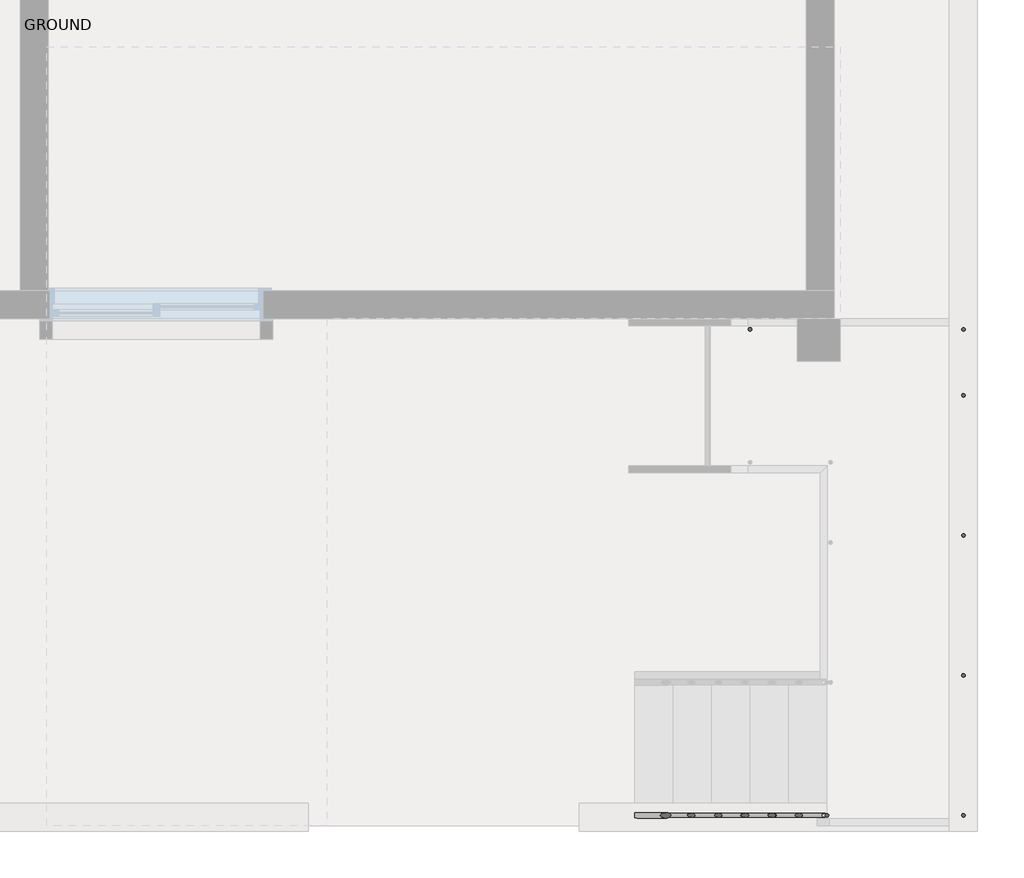
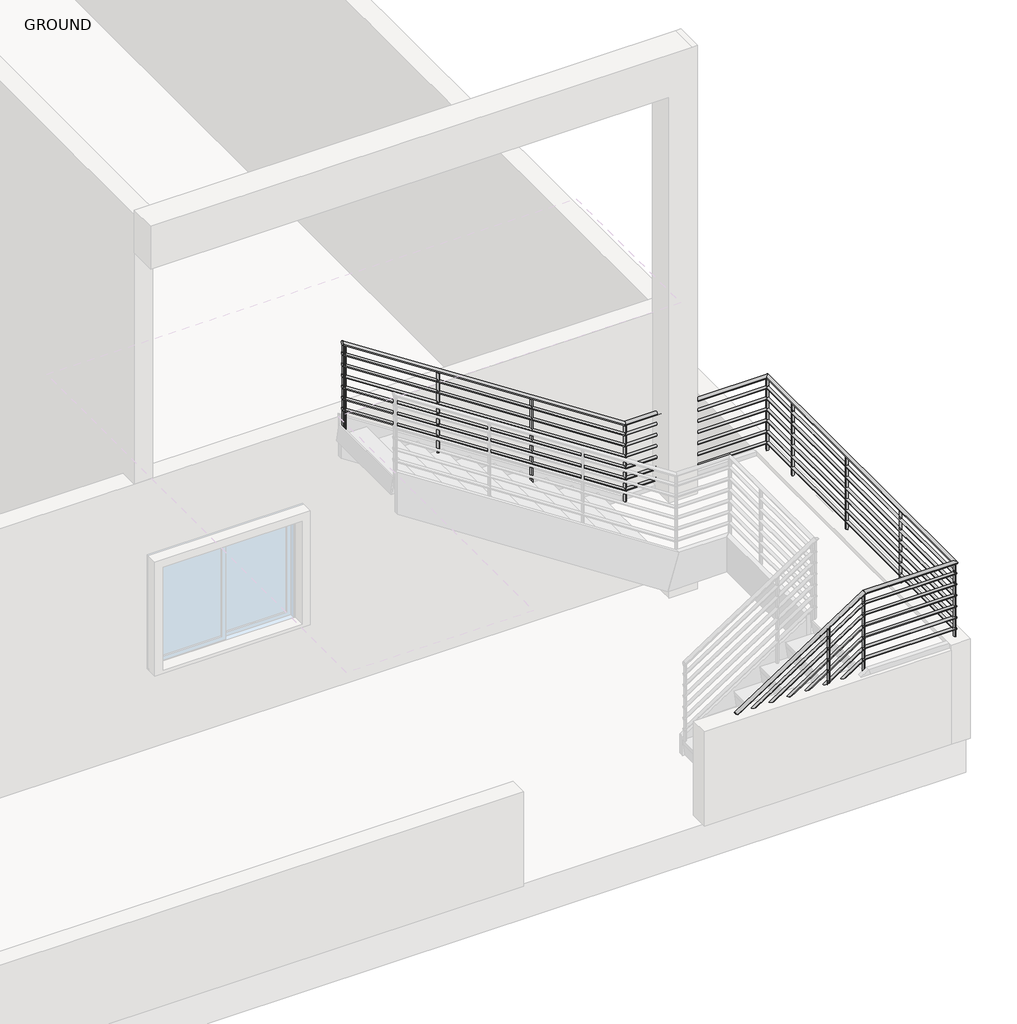
# One storey, part 2 of 4: 1 railing.
"""IFC4 building model written with IfcOpenShell, lengths in millimetres."""

from ifc_helpers import new_model, si_unit, point, frame, frame_2d, origin, place, context, project, spatial, circle_curve, ellipse_curve, trimmed, segment, composite_curve, outline, extrude, element, save
from ifc_brep_helpers import plane_surface, cylinder_surface, advanced_brep

model = new_model("IFC4")

# Units and contexts
model_context = context("Model", 3, world=origin())
ifc_project = project(units=[si_unit("LENGTHUNIT", "METRE", prefix="MILLI")], contexts=[model_context])

# Site, building, storey
site = spatial("IfcSite", under=ifc_project)
building = spatial("IfcBuilding", under=site)
storey = spatial("IfcBuildingStorey", under=building, Name="GROUND", Elevation=0.0)

# Railing
placement = place(None, origin())
element("IfcRailing", 1, ObjectType="900mm Pipe", at=placement, inside=storey, context=model_context, shape_type="SolidModel", body=[
    advanced_brep(
    [(11825.7864069, -3528.3536983, 1055.4188073), (11825.7864069, -3488.3536983, 1055.4188073), (13206.7303294, -3528.3536983, 1955.7647059), (13206.7303294, -3488.3536983, 1955.7647059), (14155.4121881, -3488.3536983, 1955.7647059), (14195.4121881, -3528.3536983, 1955.7647059), (14195.4121881, -17.2843256, 1955.7647059), (14155.4121881, -57.2843256, 1955.7647059), (12644.8424844, -17.2843256, 1955.7647059), (12644.8424844, -57.2843256, 1955.7647059), (9625.7864069, -17.2843256, 3924.1246897), (9625.7864069, -57.2843256, 3924.1246897)],
    [
        (0, 1, ellipse_curve(frame((11825.7864069, -3508.3536983, 1055.4188073), z_axis=(-1.0, 0.0, 0.0), x_axis=(0.0, 0.0, -1.0)), 23.8753103, 20.0)),
        (1, 0, ellipse_curve(frame((11825.7864069, -3508.3536983, 1055.4188073), z_axis=(-1.0, 0.0, 0.0), x_axis=(0.0, 0.0, -1.0)), 23.8753103, 20.0)),
        (0, 2),
        (2, 3, ellipse_curve(frame((13206.7303294, -3508.3536983, 1955.7647059), z_axis=(-0.9585628427581573, 0.0, -0.2848811620367351), x_axis=(0.28488116203673614, 0.0, -0.958562842758157)), 20.8645684, 20.0)),
        (3, 1),
        (3, 2, ellipse_curve(frame((13206.7303294, -3508.3536983, 1955.7647059), z_axis=(-0.9585628427581573, 0.0, -0.2848811620367351), x_axis=(0.28488116203673614, 0.0, -0.958562842758157)), 20.8645684, 20.0)),
        (4, 5, ellipse_curve(frame((14175.4121881, -3508.3536983, 1955.7647059), z_axis=(0.7071067811865513, 0.7071067811865438, 0.0), x_axis=(0.7071067811865439, -0.7071067811865512, 0.0)), 28.2842712, 20.0)),
        (5, 6),
        (6, 7, ellipse_curve(frame((14175.4121881, -37.2843256, 1955.7647059), z_axis=(0.7071067811865438, -0.7071067811865512, 0.0), x_axis=(-0.7071067811865512, -0.7071067811865438, 0.0)), 28.2842712, 20.0)),
        (7, 4),
        (5, 4, ellipse_curve(frame((14175.4121881, -3508.3536983, 1955.7647059), z_axis=(0.7071067811865513, 0.7071067811865438, 0.0), x_axis=(0.7071067811865439, -0.7071067811865512, 0.0)), 28.2842712, 20.0)),
        (7, 6, ellipse_curve(frame((14175.4121881, -37.2843256, 1955.7647059), z_axis=(0.7071067811865438, -0.7071067811865512, 0.0), x_axis=(-0.7071067811865512, -0.7071067811865438, 0.0)), 28.2842712, 20.0)),
        (6, 8),
        (8, 9, ellipse_curve(frame((12644.8424844, -37.2843256, 1955.7647059), z_axis=(0.9585628427581568, 0.0, -0.2848811620367359), x_axis=(0.2848811620367364, 0.0, 0.9585628427581568)), 20.8645684, 20.0)),
        (9, 7),
        (9, 8, ellipse_curve(frame((12644.8424844, -37.2843256, 1955.7647059), z_axis=(0.9585628427581568, 0.0, -0.2848811620367359), x_axis=(0.2848811620367364, 0.0, 0.9585628427581568)), 20.8645684, 20.0)),
        (10, 11, ellipse_curve(frame((9625.7864069, -37.2843256, 3924.1246897), z_axis=(-1.0, 0.0, 0.0), x_axis=(0.0, 0.0, -1.0)), 23.8753103, 20.0)),
        (11, 10, ellipse_curve(frame((9625.7864069, -37.2843256, 3924.1246897), z_axis=(-1.0, 0.0, 0.0), x_axis=(0.0, 0.0, -1.0)), 23.8753103, 20.0)),
        (8, 10),
        (11, 9),
        (2, 5),
        (4, 3),
    ],
    [
        plane_surface(frame((11825.7864069, -3508.3536983, 1079.2941176), z_axis=(-1.0, 0.0, 0.0), x_axis=(0.0, 1.0, 0.0))),
        cylinder_surface(frame((11836.7094668, -3508.3536983, 1062.5404087), z_axis=(-0.8376854470331991, 0.0, -0.5461529930603598), x_axis=(0.0, 1.0, 0.0)), 20.0),
        cylinder_surface(frame((14175.4121881, -3508.3536983, 1955.7647059), z_axis=(0.0, -1.0, 0.0), x_axis=(-1.0, 0.0, 0.0)), 20.0),
        cylinder_surface(frame((14175.4121881, -37.2843256, 1955.7647059), z_axis=(1.0, 0.0, 0.0), x_axis=(0.0, -1.0, 0.0)), 20.0),
        plane_surface(frame((9625.7864069, -37.2843256, 3948.0), z_axis=(-1.0, 0.0, 0.0), x_axis=(0.0, -1.0, 0.0))),
        cylinder_surface(frame((12639.863347, -37.2843256, 1959.0109969), z_axis=(0.8376854470331981, 0.0, -0.5461529930603612), x_axis=(0.0, -1.0, 0.0)), 20.0),
        cylinder_surface(frame((13200.7864069, -3508.3536983, 1955.7647059), z_axis=(-1.0, 0.0, 0.0), x_axis=(0.0, 1.0, 0.0)), 20.0),
    ],
    [
        (0, [[1, 2]]),
        (1, [[-1, 3, 4, 5]]),
        (1, [[-2, -5, 6, -3]]),
        (2, [[7, 8, 9, 10]]),
        (2, [[11, -10, 12, -8]]),
        (3, [[-9, 13, 14, 15]]),
        (3, [[-12, -15, 16, -13]]),
        (4, [[17, 18]]),
        (5, [[-14, 19, -18, 20]]),
        (5, [[-16, -20, -17, -19]]),
        (6, [[-4, 21, -7, 22]]),
        (6, [[-6, -22, -11, -21]]),
    ],
),
    advanced_brep(
    [(11825.7864069, -3493.3536983, 936.3876349), (11825.7864069, -3523.3536983, 936.3876349), (13205.2443488, -3493.3536983, 1835.7647059), (13205.2443488, -3523.3536983, 1835.7647059), (14160.4121881, -3493.3536983, 1835.7647059), (14190.4121881, -3523.3536983, 1835.7647059), (14160.4121881, -52.2843256, 1835.7647059), (14190.4121881, -22.2843256, 1835.7647059), (12646.328465, -52.2843256, 1835.7647059), (12646.328465, -22.2843256, 1835.7647059), (9625.7864069, -52.2843256, 3805.0935173), (9625.7864069, -22.2843256, 3805.0935173)],
    [
        (0, 1, ellipse_curve(frame((11825.7864069, -3508.3536983, 936.3876349), z_axis=(-1.0, 0.0, 0.0), x_axis=(0.0, 0.0, -1.0)), 17.9064827, 15.0)),
        (1, 0, ellipse_curve(frame((11825.7864069, -3508.3536983, 936.3876349), z_axis=(-1.0, 0.0, 0.0), x_axis=(0.0, 0.0, -1.0)), 17.9064827, 15.0)),
        (0, 2),
        (2, 3, ellipse_curve(frame((13205.2443488, -3508.3536983, 1835.7647059), z_axis=(-0.958562842758157, 0.0, -0.28488116203673564), x_axis=(0.28488116203673586, 0.0, -0.958562842758157)), 15.6484263, 15.0)),
        (3, 1),
        (3, 2, ellipse_curve(frame((13205.2443488, -3508.3536983, 1835.7647059), z_axis=(-0.958562842758157, 0.0, -0.28488116203673564), x_axis=(0.28488116203673586, 0.0, -0.958562842758157)), 15.6484263, 15.0)),
        (2, 4),
        (4, 5, ellipse_curve(frame((14175.4121881, -3508.3536983, 1835.7647059), z_axis=(-0.7071067811865513, -0.7071067811865438, 0.0), x_axis=(-0.7071067811865437, 0.7071067811865513, 0.0)), 21.2132034, 15.0)),
        (5, 3),
        (5, 4, ellipse_curve(frame((14175.4121881, -3508.3536983, 1835.7647059), z_axis=(-0.7071067811865513, -0.7071067811865438, 0.0), x_axis=(-0.7071067811865437, 0.7071067811865513, 0.0)), 21.2132034, 15.0)),
        (4, 6),
        (6, 7, ellipse_curve(frame((14175.4121881, -37.2843256, 1835.7647059), z_axis=(0.7071067811865438, -0.7071067811865512, 0.0), x_axis=(-0.7071067811865512, -0.7071067811865438, 0.0)), 21.2132034, 15.0)),
        (7, 5),
        (7, 6, ellipse_curve(frame((14175.4121881, -37.2843256, 1835.7647059), z_axis=(0.7071067811865438, -0.7071067811865512, 0.0), x_axis=(-0.7071067811865512, -0.7071067811865438, 0.0)), 21.2132034, 15.0)),
        (6, 8),
        (8, 9, ellipse_curve(frame((12646.328465, -37.2843256, 1835.7647059), z_axis=(0.958562842758157, 0.0, -0.2848811620367359), x_axis=(0.2848811620367357, 0.0, 0.958562842758157)), 15.6484263, 15.0)),
        (9, 7),
        (9, 8, ellipse_curve(frame((12646.328465, -37.2843256, 1835.7647059), z_axis=(0.958562842758157, 0.0, -0.2848811620367359), x_axis=(0.2848811620367357, 0.0, 0.958562842758157)), 15.6484263, 15.0)),
        (10, 11, ellipse_curve(frame((9625.7864069, -37.2843256, 3805.0935173), z_axis=(-1.0, 0.0, 0.0), x_axis=(0.0, 0.0, -1.0)), 17.9064827, 15.0)),
        (11, 10, ellipse_curve(frame((9625.7864069, -37.2843256, 3805.0935173), z_axis=(-1.0, 0.0, 0.0), x_axis=(0.0, 0.0, -1.0)), 17.9064827, 15.0)),
        (8, 10),
        (11, 9),
    ],
    [
        plane_surface(frame((11825.7864069, -3508.3536983, 954.2941176), z_axis=(-1.0, 0.0, 0.0), x_axis=(0.0, 1.0, 0.0))),
        cylinder_surface(frame((11833.9787018, -3508.3536983, 941.7288359), z_axis=(-0.8376854470331985, 0.0, -0.5461529930603609), x_axis=(0.0, -1.0, 0.0)), 15.0),
        cylinder_surface(frame((13200.7864069, -3508.3536983, 1835.7647059), z_axis=(-1.0, 0.0, 0.0), x_axis=(0.0, -1.0, 0.0)), 15.0),
        cylinder_surface(frame((14175.4121881, -3508.3536983, 1835.7647059), z_axis=(0.0, -1.0, 0.0), x_axis=(1.0, 0.0, 0.0)), 15.0),
        cylinder_surface(frame((14175.4121881, -37.2843256, 1835.7647059), z_axis=(1.0, 0.0, 0.0), x_axis=(0.0, 1.0, 0.0)), 15.0),
        plane_surface(frame((9625.7864069, -37.2843256, 3823.0), z_axis=(-1.0, 0.0, 0.0), x_axis=(0.0, -1.0, 0.0))),
        cylinder_surface(frame((12642.594112, -37.2843256, 1838.1994242), z_axis=(0.8376854470331982, 0.0, -0.5461529930603612), x_axis=(0.0, 1.0, 0.0)), 15.0),
    ],
    [
        (0, [[1, 2]]),
        (1, [[-1, 3, 4, 5]]),
        (1, [[-2, -5, 6, -3]]),
        (2, [[-4, 7, 8, 9]]),
        (2, [[-6, -9, 10, -7]]),
        (3, [[-8, 11, 12, 13]]),
        (3, [[-10, -13, 14, -11]]),
        (4, [[-12, 15, 16, 17]]),
        (4, [[-14, -17, 18, -15]]),
        (5, [[19, 20]]),
        (6, [[-16, 21, -20, 22]]),
        (6, [[-18, -22, -19, -21]]),
    ],
),
    advanced_brep(
    [(11825.7864069, -3493.3536983, 811.3876349), (11825.7864069, -3523.3536983, 811.3876349), (13205.2443488, -3493.3536983, 1710.7647059), (13205.2443488, -3523.3536983, 1710.7647059), (14160.4121881, -3493.3536983, 1710.7647059), (14190.4121881, -3523.3536983, 1710.7647059), (14160.4121881, -52.2843256, 1710.7647059), (14190.4121881, -22.2843256, 1710.7647059), (12646.328465, -52.2843256, 1710.7647059), (12646.328465, -22.2843256, 1710.7647059), (9625.7864069, -52.2843256, 3680.0935173), (9625.7864069, -22.2843256, 3680.0935173)],
    [
        (0, 1, ellipse_curve(frame((11825.7864069, -3508.3536983, 811.3876349), z_axis=(-1.0, 0.0, 0.0), x_axis=(0.0, 0.0, -1.0)), 17.9064827, 15.0)),
        (1, 0, ellipse_curve(frame((11825.7864069, -3508.3536983, 811.3876349), z_axis=(-1.0, 0.0, 0.0), x_axis=(0.0, 0.0, -1.0)), 17.9064827, 15.0)),
        (0, 2),
        (2, 3, ellipse_curve(frame((13205.2443488, -3508.3536983, 1710.7647059), z_axis=(-0.958562842758157, 0.0, -0.28488116203673564), x_axis=(0.28488116203673586, 0.0, -0.958562842758157)), 15.6484263, 15.0)),
        (3, 1),
        (3, 2, ellipse_curve(frame((13205.2443488, -3508.3536983, 1710.7647059), z_axis=(-0.958562842758157, 0.0, -0.28488116203673564), x_axis=(0.28488116203673586, 0.0, -0.958562842758157)), 15.6484263, 15.0)),
        (2, 4),
        (4, 5, ellipse_curve(frame((14175.4121881, -3508.3536983, 1710.7647059), z_axis=(-0.7071067811865513, -0.7071067811865438, 0.0), x_axis=(-0.7071067811865437, 0.7071067811865513, 0.0)), 21.2132034, 15.0)),
        (5, 3),
        (5, 4, ellipse_curve(frame((14175.4121881, -3508.3536983, 1710.7647059), z_axis=(-0.7071067811865513, -0.7071067811865438, 0.0), x_axis=(-0.7071067811865437, 0.7071067811865513, 0.0)), 21.2132034, 15.0)),
        (4, 6),
        (6, 7, ellipse_curve(frame((14175.4121881, -37.2843256, 1710.7647059), z_axis=(0.7071067811865438, -0.7071067811865512, 0.0), x_axis=(-0.7071067811865512, -0.7071067811865438, 0.0)), 21.2132034, 15.0)),
        (7, 5),
        (7, 6, ellipse_curve(frame((14175.4121881, -37.2843256, 1710.7647059), z_axis=(0.7071067811865438, -0.7071067811865512, 0.0), x_axis=(-0.7071067811865512, -0.7071067811865438, 0.0)), 21.2132034, 15.0)),
        (6, 8),
        (8, 9, ellipse_curve(frame((12646.328465, -37.2843256, 1710.7647059), z_axis=(0.9585628427581568, 0.0, -0.2848811620367359), x_axis=(0.28488116203673647, 0.0, 0.9585628427581567)), 15.6484263, 15.0)),
        (9, 7),
        (9, 8, ellipse_curve(frame((12646.328465, -37.2843256, 1710.7647059), z_axis=(0.9585628427581568, 0.0, -0.2848811620367359), x_axis=(0.28488116203673647, 0.0, 0.9585628427581567)), 15.6484263, 15.0)),
        (10, 11, ellipse_curve(frame((9625.7864069, -37.2843256, 3680.0935173), z_axis=(-1.0, 0.0, 0.0), x_axis=(0.0, 0.0, -1.0)), 17.9064827, 15.0)),
        (11, 10, ellipse_curve(frame((9625.7864069, -37.2843256, 3680.0935173), z_axis=(-1.0, 0.0, 0.0), x_axis=(0.0, 0.0, -1.0)), 17.9064827, 15.0)),
        (8, 10),
        (11, 9),
    ],
    [
        plane_surface(frame((11825.7864069, -3508.3536983, 829.2941176), z_axis=(-1.0, 0.0, 0.0), x_axis=(0.0, 1.0, 0.0))),
        cylinder_surface(frame((11833.9787018, -3508.3536983, 816.7288359), z_axis=(-0.8376854470331985, 0.0, -0.5461529930603609), x_axis=(0.0, -1.0, 0.0)), 15.0),
        cylinder_surface(frame((13200.7864069, -3508.3536983, 1710.7647059), z_axis=(-1.0, 0.0, 0.0), x_axis=(0.0, -1.0, 0.0)), 15.0),
        cylinder_surface(frame((14175.4121881, -3508.3536983, 1710.7647059), z_axis=(0.0, -1.0, 0.0), x_axis=(1.0, 0.0, 0.0)), 15.0),
        cylinder_surface(frame((14175.4121881, -37.2843256, 1710.7647059), z_axis=(1.0, 0.0, 0.0), x_axis=(0.0, 1.0, 0.0)), 15.0),
        plane_surface(frame((9625.7864069, -37.2843256, 3698.0), z_axis=(-1.0, 0.0, 0.0), x_axis=(0.0, -1.0, 0.0))),
        cylinder_surface(frame((12642.594112, -37.2843256, 1713.1994242), z_axis=(0.8376854470331981, 0.0, -0.5461529930603612), x_axis=(0.0, 1.0, 0.0)), 15.0),
    ],
    [
        (0, [[1, 2]]),
        (1, [[-1, 3, 4, 5]]),
        (1, [[-2, -5, 6, -3]]),
        (2, [[-4, 7, 8, 9]]),
        (2, [[-6, -9, 10, -7]]),
        (3, [[-8, 11, 12, 13]]),
        (3, [[-10, -13, 14, -11]]),
        (4, [[-12, 15, 16, 17]]),
        (4, [[-14, -17, 18, -15]]),
        (5, [[19, 20]]),
        (6, [[-16, 21, -20, 22]]),
        (6, [[-18, -22, -19, -21]]),
    ],
),
    advanced_brep(
    [(11825.7864069, -3493.3536983, 686.3876349), (11825.7864069, -3523.3536983, 686.3876349), (13205.2443488, -3493.3536983, 1585.7647059), (13205.2443488, -3523.3536983, 1585.7647059), (14160.4121881, -3493.3536983, 1585.7647059), (14190.4121881, -3523.3536983, 1585.7647059), (14160.4121881, -52.2843256, 1585.7647059), (14190.4121881, -22.2843256, 1585.7647059), (12646.328465, -52.2843256, 1585.7647059), (12646.328465, -22.2843256, 1585.7647059), (9625.7864069, -52.2843256, 3555.0935173), (9625.7864069, -22.2843256, 3555.0935173)],
    [
        (0, 1, ellipse_curve(frame((11825.7864069, -3508.3536983, 686.3876349), z_axis=(-1.0, 0.0, 0.0), x_axis=(0.0, 0.0, -1.0)), 17.9064827, 15.0)),
        (1, 0, ellipse_curve(frame((11825.7864069, -3508.3536983, 686.3876349), z_axis=(-1.0, 0.0, 0.0), x_axis=(0.0, 0.0, -1.0)), 17.9064827, 15.0)),
        (0, 2),
        (2, 3, ellipse_curve(frame((13205.2443488, -3508.3536983, 1585.7647059), z_axis=(-0.958562842758157, 0.0, -0.28488116203673564), x_axis=(0.28488116203673586, 0.0, -0.958562842758157)), 15.6484263, 15.0)),
        (3, 1),
        (3, 2, ellipse_curve(frame((13205.2443488, -3508.3536983, 1585.7647059), z_axis=(-0.958562842758157, 0.0, -0.28488116203673564), x_axis=(0.28488116203673586, 0.0, -0.958562842758157)), 15.6484263, 15.0)),
        (2, 4),
        (4, 5, ellipse_curve(frame((14175.4121881, -3508.3536983, 1585.7647059), z_axis=(-0.7071067811865513, -0.7071067811865438, 0.0), x_axis=(-0.7071067811865437, 0.7071067811865513, 0.0)), 21.2132034, 15.0)),
        (5, 3),
        (5, 4, ellipse_curve(frame((14175.4121881, -3508.3536983, 1585.7647059), z_axis=(-0.7071067811865513, -0.7071067811865438, 0.0), x_axis=(-0.7071067811865437, 0.7071067811865513, 0.0)), 21.2132034, 15.0)),
        (4, 6),
        (6, 7, ellipse_curve(frame((14175.4121881, -37.2843256, 1585.7647059), z_axis=(0.7071067811865438, -0.7071067811865512, 0.0), x_axis=(-0.7071067811865512, -0.7071067811865438, 0.0)), 21.2132034, 15.0)),
        (7, 5),
        (7, 6, ellipse_curve(frame((14175.4121881, -37.2843256, 1585.7647059), z_axis=(0.7071067811865438, -0.7071067811865512, 0.0), x_axis=(-0.7071067811865512, -0.7071067811865438, 0.0)), 21.2132034, 15.0)),
        (6, 8),
        (8, 9, ellipse_curve(frame((12646.328465, -37.2843256, 1585.7647059), z_axis=(0.958562842758157, 0.0, -0.28488116203673575), x_axis=(0.28488116203673586, 0.0, 0.958562842758157)), 15.6484263, 15.0)),
        (9, 7),
        (9, 8, ellipse_curve(frame((12646.328465, -37.2843256, 1585.7647059), z_axis=(0.958562842758157, 0.0, -0.28488116203673575), x_axis=(0.28488116203673586, 0.0, 0.958562842758157)), 15.6484263, 15.0)),
        (10, 11, ellipse_curve(frame((9625.7864069, -37.2843256, 3555.0935173), z_axis=(-1.0, 0.0, 0.0), x_axis=(0.0, 0.0, -1.0)), 17.9064827, 15.0)),
        (11, 10, ellipse_curve(frame((9625.7864069, -37.2843256, 3555.0935173), z_axis=(-1.0, 0.0, 0.0), x_axis=(0.0, 0.0, -1.0)), 17.9064827, 15.0)),
        (8, 10),
        (11, 9),
    ],
    [
        plane_surface(frame((11825.7864069, -3508.3536983, 704.2941176), z_axis=(-1.0, 0.0, 0.0), x_axis=(0.0, 1.0, 0.0))),
        cylinder_surface(frame((11833.9787018, -3508.3536983, 691.7288359), z_axis=(-0.8376854470331985, 0.0, -0.5461529930603609), x_axis=(0.0, -1.0, 0.0)), 15.0),
        cylinder_surface(frame((13200.7864069, -3508.3536983, 1585.7647059), z_axis=(-1.0, 0.0, 0.0), x_axis=(0.0, -1.0, 0.0)), 15.0),
        cylinder_surface(frame((14175.4121881, -3508.3536983, 1585.7647059), z_axis=(0.0, -1.0, 0.0), x_axis=(1.0, 0.0, 0.0)), 15.0),
        cylinder_surface(frame((14175.4121881, -37.2843256, 1585.7647059), z_axis=(1.0, 0.0, 0.0), x_axis=(0.0, 1.0, 0.0)), 15.0),
        plane_surface(frame((9625.7864069, -37.2843256, 3573.0), z_axis=(-1.0, 0.0, 0.0), x_axis=(0.0, -1.0, 0.0))),
        cylinder_surface(frame((12642.594112, -37.2843256, 1588.1994242), z_axis=(0.8376854470331982, 0.0, -0.546152993060361), x_axis=(0.0, 1.0, 0.0)), 15.0),
    ],
    [
        (0, [[1, 2]]),
        (1, [[-1, 3, 4, 5]]),
        (1, [[-2, -5, 6, -3]]),
        (2, [[-4, 7, 8, 9]]),
        (2, [[-6, -9, 10, -7]]),
        (3, [[-8, 11, 12, 13]]),
        (3, [[-10, -13, 14, -11]]),
        (4, [[-12, 15, 16, 17]]),
        (4, [[-14, -17, 18, -15]]),
        (5, [[19, 20]]),
        (6, [[-16, 21, -20, 22]]),
        (6, [[-18, -22, -19, -21]]),
    ],
),
    advanced_brep(
    [(11825.7864069, -3493.3536983, 561.3876349), (11825.7864069, -3523.3536983, 561.3876349), (13205.2443488, -3493.3536983, 1460.7647059), (13205.2443488, -3523.3536983, 1460.7647059), (14160.4121881, -3493.3536983, 1460.7647059), (14190.4121881, -3523.3536983, 1460.7647059), (14160.4121881, -52.2843256, 1460.7647059), (14190.4121881, -22.2843256, 1460.7647059), (12646.328465, -52.2843256, 1460.7647059), (12646.328465, -22.2843256, 1460.7647059), (9625.7864069, -52.2843256, 3430.0935173), (9625.7864069, -22.2843256, 3430.0935173)],
    [
        (0, 1, ellipse_curve(frame((11825.7864069, -3508.3536983, 561.3876349), z_axis=(-1.0, 0.0, 0.0), x_axis=(0.0, 0.0, -1.0)), 17.9064827, 15.0)),
        (1, 0, ellipse_curve(frame((11825.7864069, -3508.3536983, 561.3876349), z_axis=(-1.0, 0.0, 0.0), x_axis=(0.0, 0.0, -1.0)), 17.9064827, 15.0)),
        (0, 2),
        (2, 3, ellipse_curve(frame((13205.2443488, -3508.3536983, 1460.7647059), z_axis=(-0.958562842758157, 0.0, -0.28488116203673564), x_axis=(0.28488116203673586, 0.0, -0.958562842758157)), 15.6484263, 15.0)),
        (3, 1),
        (3, 2, ellipse_curve(frame((13205.2443488, -3508.3536983, 1460.7647059), z_axis=(-0.958562842758157, 0.0, -0.28488116203673564), x_axis=(0.28488116203673586, 0.0, -0.958562842758157)), 15.6484263, 15.0)),
        (2, 4),
        (4, 5, ellipse_curve(frame((14175.4121881, -3508.3536983, 1460.7647059), z_axis=(-0.7071067811865513, -0.7071067811865438, 0.0), x_axis=(-0.7071067811865437, 0.7071067811865513, 0.0)), 21.2132034, 15.0)),
        (5, 3),
        (5, 4, ellipse_curve(frame((14175.4121881, -3508.3536983, 1460.7647059), z_axis=(-0.7071067811865513, -0.7071067811865438, 0.0), x_axis=(-0.7071067811865437, 0.7071067811865513, 0.0)), 21.2132034, 15.0)),
        (4, 6),
        (6, 7, ellipse_curve(frame((14175.4121881, -37.2843256, 1460.7647059), z_axis=(0.7071067811865438, -0.7071067811865512, 0.0), x_axis=(-0.7071067811865512, -0.7071067811865438, 0.0)), 21.2132034, 15.0)),
        (7, 5),
        (7, 6, ellipse_curve(frame((14175.4121881, -37.2843256, 1460.7647059), z_axis=(0.7071067811865438, -0.7071067811865512, 0.0), x_axis=(-0.7071067811865512, -0.7071067811865438, 0.0)), 21.2132034, 15.0)),
        (6, 8),
        (8, 9, ellipse_curve(frame((12646.328465, -37.2843256, 1460.7647059), z_axis=(0.9585628427581568, 0.0, -0.2848811620367359), x_axis=(0.28488116203673647, 0.0, 0.9585628427581567)), 15.6484263, 15.0)),
        (9, 7),
        (9, 8, ellipse_curve(frame((12646.328465, -37.2843256, 1460.7647059), z_axis=(0.9585628427581568, 0.0, -0.2848811620367359), x_axis=(0.28488116203673647, 0.0, 0.9585628427581567)), 15.6484263, 15.0)),
        (10, 11, ellipse_curve(frame((9625.7864069, -37.2843256, 3430.0935173), z_axis=(-1.0, 0.0, 0.0), x_axis=(0.0, 0.0, -1.0)), 17.9064827, 15.0)),
        (11, 10, ellipse_curve(frame((9625.7864069, -37.2843256, 3430.0935173), z_axis=(-1.0, 0.0, 0.0), x_axis=(0.0, 0.0, -1.0)), 17.9064827, 15.0)),
        (8, 10),
        (11, 9),
    ],
    [
        plane_surface(frame((11825.7864069, -3508.3536983, 579.2941176), z_axis=(-1.0, 0.0, 0.0), x_axis=(0.0, 1.0, 0.0))),
        cylinder_surface(frame((11833.9787018, -3508.3536983, 566.7288359), z_axis=(-0.8376854470331985, 0.0, -0.5461529930603609), x_axis=(0.0, -1.0, 0.0)), 15.0),
        cylinder_surface(frame((13200.7864069, -3508.3536983, 1460.7647059), z_axis=(-1.0, 0.0, 0.0), x_axis=(0.0, -1.0, 0.0)), 15.0),
        cylinder_surface(frame((14175.4121881, -3508.3536983, 1460.7647059), z_axis=(0.0, -1.0, 0.0), x_axis=(1.0, 0.0, 0.0)), 15.0),
        cylinder_surface(frame((14175.4121881, -37.2843256, 1460.7647059), z_axis=(1.0, 0.0, 0.0), x_axis=(0.0, 1.0, 0.0)), 15.0),
        plane_surface(frame((9625.7864069, -37.2843256, 3448.0), z_axis=(-1.0, 0.0, 0.0), x_axis=(0.0, -1.0, 0.0))),
        cylinder_surface(frame((12642.594112, -37.2843256, 1463.1994242), z_axis=(0.8376854470331981, 0.0, -0.5461529930603612), x_axis=(0.0, 1.0, 0.0)), 15.0),
    ],
    [
        (0, [[1, 2]]),
        (1, [[-1, 3, 4, 5]]),
        (1, [[-2, -5, 6, -3]]),
        (2, [[-4, 7, 8, 9]]),
        (2, [[-6, -9, 10, -7]]),
        (3, [[-8, 11, 12, 13]]),
        (3, [[-10, -13, 14, -11]]),
        (4, [[-12, 15, 16, 17]]),
        (4, [[-14, -17, 18, -15]]),
        (5, [[19, 20]]),
        (6, [[-16, 21, -20, 22]]),
        (6, [[-18, -22, -19, -21]]),
    ],
),
    advanced_brep(
    [(11825.7864069, -3493.3536983, 436.3876349), (11825.7864069, -3523.3536983, 436.3876349), (13205.2443488, -3493.3536983, 1335.7647059), (13205.2443488, -3523.3536983, 1335.7647059), (14160.4121881, -3493.3536983, 1335.7647059), (14190.4121881, -3523.3536983, 1335.7647059), (14160.4121881, -52.2843256, 1335.7647059), (14190.4121881, -22.2843256, 1335.7647059), (12646.328465, -52.2843256, 1335.7647059), (12646.328465, -22.2843256, 1335.7647059), (9625.7864069, -52.2843256, 3305.0935173), (9625.7864069, -22.2843256, 3305.0935173)],
    [
        (0, 1, ellipse_curve(frame((11825.7864069, -3508.3536983, 436.3876349), z_axis=(-1.0, 0.0, 0.0), x_axis=(0.0, 0.0, -1.0)), 17.9064827, 15.0)),
        (1, 0, ellipse_curve(frame((11825.7864069, -3508.3536983, 436.3876349), z_axis=(-1.0, 0.0, 0.0), x_axis=(0.0, 0.0, -1.0)), 17.9064827, 15.0)),
        (0, 2),
        (2, 3, ellipse_curve(frame((13205.2443488, -3508.3536983, 1335.7647059), z_axis=(-0.958562842758157, 0.0, -0.28488116203673564), x_axis=(0.28488116203673586, 0.0, -0.958562842758157)), 15.6484263, 15.0)),
        (3, 1),
        (3, 2, ellipse_curve(frame((13205.2443488, -3508.3536983, 1335.7647059), z_axis=(-0.958562842758157, 0.0, -0.28488116203673564), x_axis=(0.28488116203673586, 0.0, -0.958562842758157)), 15.6484263, 15.0)),
        (2, 4),
        (4, 5, ellipse_curve(frame((14175.4121881, -3508.3536983, 1335.7647059), z_axis=(-0.7071067811865513, -0.7071067811865438, 0.0), x_axis=(-0.7071067811865437, 0.7071067811865513, 0.0)), 21.2132034, 15.0)),
        (5, 3),
        (5, 4, ellipse_curve(frame((14175.4121881, -3508.3536983, 1335.7647059), z_axis=(-0.7071067811865513, -0.7071067811865438, 0.0), x_axis=(-0.7071067811865437, 0.7071067811865513, 0.0)), 21.2132034, 15.0)),
        (4, 6),
        (6, 7, ellipse_curve(frame((14175.4121881, -37.2843256, 1335.7647059), z_axis=(0.7071067811865438, -0.7071067811865512, 0.0), x_axis=(-0.7071067811865512, -0.7071067811865438, 0.0)), 21.2132034, 15.0)),
        (7, 5),
        (7, 6, ellipse_curve(frame((14175.4121881, -37.2843256, 1335.7647059), z_axis=(0.7071067811865438, -0.7071067811865512, 0.0), x_axis=(-0.7071067811865512, -0.7071067811865438, 0.0)), 21.2132034, 15.0)),
        (6, 8),
        (8, 9, ellipse_curve(frame((12646.328465, -37.2843256, 1335.7647059), z_axis=(0.958562842758157, 0.0, -0.2848811620367359), x_axis=(0.2848811620367357, 0.0, 0.958562842758157)), 15.6484263, 15.0)),
        (9, 7),
        (9, 8, ellipse_curve(frame((12646.328465, -37.2843256, 1335.7647059), z_axis=(0.958562842758157, 0.0, -0.2848811620367359), x_axis=(0.2848811620367357, 0.0, 0.958562842758157)), 15.6484263, 15.0)),
        (10, 11, ellipse_curve(frame((9625.7864069, -37.2843256, 3305.0935173), z_axis=(-1.0, 0.0, 0.0), x_axis=(0.0, 0.0, -1.0)), 17.9064827, 15.0)),
        (11, 10, ellipse_curve(frame((9625.7864069, -37.2843256, 3305.0935173), z_axis=(-1.0, 0.0, 0.0), x_axis=(0.0, 0.0, -1.0)), 17.9064827, 15.0)),
        (8, 10),
        (11, 9),
    ],
    [
        plane_surface(frame((11825.7864069, -3508.3536983, 454.2941176), z_axis=(-1.0, 0.0, 0.0), x_axis=(0.0, 1.0, 0.0))),
        cylinder_surface(frame((11833.9787018, -3508.3536983, 441.7288359), z_axis=(-0.8376854470331985, 0.0, -0.5461529930603609), x_axis=(0.0, -1.0, 0.0)), 15.0),
        cylinder_surface(frame((13200.7864069, -3508.3536983, 1335.7647059), z_axis=(-1.0, 0.0, 0.0), x_axis=(0.0, -1.0, 0.0)), 15.0),
        cylinder_surface(frame((14175.4121881, -3508.3536983, 1335.7647059), z_axis=(0.0, -1.0, 0.0), x_axis=(1.0, 0.0, 0.0)), 15.0),
        cylinder_surface(frame((14175.4121881, -37.2843256, 1335.7647059), z_axis=(1.0, 0.0, 0.0), x_axis=(0.0, 1.0, 0.0)), 15.0),
        plane_surface(frame((9625.7864069, -37.2843256, 3323.0), z_axis=(-1.0, 0.0, 0.0), x_axis=(0.0, -1.0, 0.0))),
        cylinder_surface(frame((12642.594112, -37.2843256, 1338.1994242), z_axis=(0.8376854470331982, 0.0, -0.5461529930603612), x_axis=(0.0, 1.0, 0.0)), 15.0),
    ],
    [
        (0, [[1, 2]]),
        (1, [[-1, 3, 4, 5]]),
        (1, [[-2, -5, 6, -3]]),
        (2, [[-4, 7, 8, 9]]),
        (2, [[-6, -9, 10, -7]]),
        (3, [[-8, 11, 12, 13]]),
        (3, [[-10, -13, 14, -11]]),
        (4, [[-12, 15, 16, 17]]),
        (4, [[-14, -17, 18, -15]]),
        (5, [[19, 20]]),
        (6, [[-16, 21, -20, 22]]),
        (6, [[-18, -22, -19, -21]]),
    ],
),
    advanced_brep(
    [(11825.7864069, -3493.3536983, 311.3876349), (11825.7864069, -3523.3536983, 311.3876349), (13205.2443488, -3493.3536983, 1210.7647059), (13205.2443488, -3523.3536983, 1210.7647059), (14160.4121881, -3493.3536983, 1210.7647059), (14190.4121881, -3523.3536983, 1210.7647059), (14160.4121881, -52.2843256, 1210.7647059), (14190.4121881, -22.2843256, 1210.7647059), (12646.328465, -52.2843256, 1210.7647059), (12646.328465, -22.2843256, 1210.7647059), (9625.7864069, -52.2843256, 3180.0935173), (9625.7864069, -22.2843256, 3180.0935173)],
    [
        (0, 1, ellipse_curve(frame((11825.7864069, -3508.3536983, 311.3876349), z_axis=(-1.0, 0.0, 0.0), x_axis=(0.0, 0.0, -1.0)), 17.9064827, 15.0)),
        (1, 0, ellipse_curve(frame((11825.7864069, -3508.3536983, 311.3876349), z_axis=(-1.0, 0.0, 0.0), x_axis=(0.0, 0.0, -1.0)), 17.9064827, 15.0)),
        (0, 2),
        (2, 3, ellipse_curve(frame((13205.2443488, -3508.3536983, 1210.7647059), z_axis=(-0.958562842758157, 0.0, -0.28488116203673564), x_axis=(0.28488116203673586, 0.0, -0.958562842758157)), 15.6484263, 15.0)),
        (3, 1),
        (3, 2, ellipse_curve(frame((13205.2443488, -3508.3536983, 1210.7647059), z_axis=(-0.958562842758157, 0.0, -0.28488116203673564), x_axis=(0.28488116203673586, 0.0, -0.958562842758157)), 15.6484263, 15.0)),
        (2, 4),
        (4, 5, ellipse_curve(frame((14175.4121881, -3508.3536983, 1210.7647059), z_axis=(-0.7071067811865513, -0.7071067811865438, 0.0), x_axis=(-0.7071067811865437, 0.7071067811865513, 0.0)), 21.2132034, 15.0)),
        (5, 3),
        (5, 4, ellipse_curve(frame((14175.4121881, -3508.3536983, 1210.7647059), z_axis=(-0.7071067811865513, -0.7071067811865438, 0.0), x_axis=(-0.7071067811865437, 0.7071067811865513, 0.0)), 21.2132034, 15.0)),
        (4, 6),
        (6, 7, ellipse_curve(frame((14175.4121881, -37.2843256, 1210.7647059), z_axis=(0.7071067811865438, -0.7071067811865512, 0.0), x_axis=(-0.7071067811865512, -0.7071067811865438, 0.0)), 21.2132034, 15.0)),
        (7, 5),
        (7, 6, ellipse_curve(frame((14175.4121881, -37.2843256, 1210.7647059), z_axis=(0.7071067811865438, -0.7071067811865512, 0.0), x_axis=(-0.7071067811865512, -0.7071067811865438, 0.0)), 21.2132034, 15.0)),
        (6, 8),
        (8, 9, ellipse_curve(frame((12646.328465, -37.2843256, 1210.7647059), z_axis=(0.9585628427581568, 0.0, -0.2848811620367359), x_axis=(0.28488116203673647, 0.0, 0.9585628427581567)), 15.6484263, 15.0)),
        (9, 7),
        (9, 8, ellipse_curve(frame((12646.328465, -37.2843256, 1210.7647059), z_axis=(0.9585628427581568, 0.0, -0.2848811620367359), x_axis=(0.28488116203673647, 0.0, 0.9585628427581567)), 15.6484263, 15.0)),
        (10, 11, ellipse_curve(frame((9625.7864069, -37.2843256, 3180.0935173), z_axis=(-1.0, 0.0, 0.0), x_axis=(0.0, 0.0, -1.0)), 17.9064827, 15.0)),
        (11, 10, ellipse_curve(frame((9625.7864069, -37.2843256, 3180.0935173), z_axis=(-1.0, 0.0, 0.0), x_axis=(0.0, 0.0, -1.0)), 17.9064827, 15.0)),
        (8, 10),
        (11, 9),
    ],
    [
        plane_surface(frame((11825.7864069, -3508.3536983, 329.2941176), z_axis=(-1.0, 0.0, 0.0), x_axis=(0.0, 1.0, 0.0))),
        cylinder_surface(frame((11833.9787018, -3508.3536983, 316.7288359), z_axis=(-0.8376854470331985, 0.0, -0.5461529930603609), x_axis=(0.0, -1.0, 0.0)), 15.0),
        cylinder_surface(frame((13200.7864069, -3508.3536983, 1210.7647059), z_axis=(-1.0, 0.0, 0.0), x_axis=(0.0, -1.0, 0.0)), 15.0),
        cylinder_surface(frame((14175.4121881, -3508.3536983, 1210.7647059), z_axis=(0.0, -1.0, 0.0), x_axis=(1.0, 0.0, 0.0)), 15.0),
        cylinder_surface(frame((14175.4121881, -37.2843256, 1210.7647059), z_axis=(1.0, 0.0, 0.0), x_axis=(0.0, 1.0, 0.0)), 15.0),
        plane_surface(frame((9625.7864069, -37.2843256, 3198.0), z_axis=(-1.0, 0.0, 0.0), x_axis=(0.0, -1.0, 0.0))),
        cylinder_surface(frame((12642.594112, -37.2843256, 1213.1994242), z_axis=(0.8376854470331981, 0.0, -0.5461529930603612), x_axis=(0.0, 1.0, 0.0)), 15.0),
    ],
    [
        (0, [[1, 2]]),
        (1, [[-1, 3, 4, 5]]),
        (1, [[-2, -5, 6, -3]]),
        (2, [[-4, 7, 8, 9]]),
        (2, [[-6, -9, 10, -7]]),
        (3, [[-8, 11, 12, 13]]),
        (3, [[-10, -13, 14, -11]]),
        (4, [[-12, 15, 16, 17]]),
        (4, [[-14, -17, 18, -15]]),
        (5, [[19, 20]]),
        (6, [[-16, 21, -20, 22]]),
        (6, [[-18, -22, -19, -21]]),
    ],
),
    advanced_brep(
    [(9650.7864069, -24.7843256, 3883.9499141), (9650.7864069, -24.7843256, 2868.7058824), (9650.7864069, -49.7843256, 2868.7058824), (9650.7864069, -49.7843256, 3883.9499141)],
    [
        (0, 1),
        (1, 2, circle_curve(frame((9650.7864069, -37.2843256, 2868.7058824), z_axis=(0.0, 0.0, 1.0), x_axis=(0.0, -1.0, 0.0)), 12.5)),
        (2, 3),
        (3, 0, ellipse_curve(frame((9650.7864069, -37.2843256, 3883.9499141), z_axis=(-0.546152993060361, 0.0, -0.8376854470331982), x_axis=(-0.8376854470331982, 0.0, 0.546152993060361)), 14.922069, 12.5)),
        (0, 3, ellipse_curve(frame((9650.7864069, -37.2843256, 3883.9499141), z_axis=(-0.546152993060361, 0.0, -0.8376854470331982), x_axis=(-0.8376854470331982, 0.0, 0.546152993060361)), 14.922069, 12.5)),
        (2, 1, circle_curve(frame((9650.7864069, -37.2843256, 2868.7058824), z_axis=(0.0, 0.0, 1.0), x_axis=(0.0, -1.0, 0.0)), 12.5)),
    ],
    [
        cylinder_surface(frame((9650.7864069, -37.2843256, 2768.7058824), z_axis=(0.0, 0.0, 1.0), x_axis=(0.0, -1.0, 0.0)), 12.5),
        plane_surface(frame((9625.7864069, -62.2843256, 3900.2493794), z_axis=(0.546152993060361, 0.0, 0.8376854470331982), x_axis=(0.0, 1.0, 0.0))),
        plane_surface(frame((9675.7864069, -62.2843256, 2868.7058824), z_axis=(0.0, 0.0, -1.0), x_axis=(0.0, 1.0, 0.0))),
    ],
    [
        (0, [[1, 2, 3, 4]]),
        (0, [[-1, 5, -3, 6]]),
        (1, [[-4, -5]]),
        (2, [[-2, -6]]),
    ],
),
    advanced_brep(
    [(10650.7864069, -24.7843256, 3231.9713045), (10650.7864069, -24.7843256, 2330.8235294), (10650.7864069, -49.7843256, 2330.8235294), (10650.7864069, -49.7843256, 3231.9713045)],
    [
        (0, 1),
        (1, 2, circle_curve(frame((10650.7864069, -37.2843256, 2330.8235294), z_axis=(0.0, 0.0, 1.0), x_axis=(0.0, -1.0, 0.0)), 12.5)),
        (2, 3),
        (3, 0, ellipse_curve(frame((10650.7864069, -37.2843256, 3231.9713045), z_axis=(-0.5461529930603595, 0.0, -0.8376854470331992), x_axis=(-0.8376854470331992, 0.0, 0.5461529930603595)), 14.922069, 12.5)),
        (0, 3, ellipse_curve(frame((10650.7864069, -37.2843256, 3231.9713045), z_axis=(-0.5461529930603595, 0.0, -0.8376854470331992), x_axis=(-0.8376854470331992, 0.0, 0.5461529930603595)), 14.922069, 12.5)),
        (2, 1, circle_curve(frame((10650.7864069, -37.2843256, 2330.8235294), z_axis=(0.0, 0.0, 1.0), x_axis=(0.0, -1.0, 0.0)), 12.5)),
    ],
    [
        cylinder_surface(frame((10650.7864069, -37.2843256, 2230.8235294), z_axis=(0.0, 0.0, 1.0), x_axis=(0.0, -1.0, 0.0)), 12.5),
        plane_surface(frame((10625.7864069, -62.2843256, 3248.2707697), z_axis=(0.5461529930603595, 0.0, 0.8376854470331992), x_axis=(0.0, 1.0, 0.0))),
        plane_surface(frame((10675.7864069, -62.2843256, 2330.8235294), z_axis=(0.0, 0.0, -1.0), x_axis=(0.0, 1.0, 0.0))),
    ],
    [
        (0, [[1, 2, 3, 4]]),
        (0, [[-1, 5, -3, 6]]),
        (1, [[-4, -5]]),
        (2, [[-2, -6]]),
    ],
),
    advanced_brep(
    [(11650.7864069, -24.7843256, 2579.9926949), (11650.7864069, -24.7843256, 1613.6470588), (11650.7864069, -49.7843256, 1613.6470588), (11650.7864069, -49.7843256, 2579.9926949)],
    [
        (0, 1),
        (1, 2, circle_curve(frame((11650.7864069, -37.2843256, 1613.6470588), z_axis=(0.0, 0.0, 1.0), x_axis=(0.0, -1.0, 0.0)), 12.5)),
        (2, 3),
        (3, 0, ellipse_curve(frame((11650.7864069, -37.2843256, 2579.9926949), z_axis=(-0.5461529930603595, 0.0, -0.8376854470331992), x_axis=(-0.8376854470331992, 0.0, 0.5461529930603595)), 14.922069, 12.5)),
        (0, 3, ellipse_curve(frame((11650.7864069, -37.2843256, 2579.9926949), z_axis=(-0.5461529930603595, 0.0, -0.8376854470331992), x_axis=(-0.8376854470331992, 0.0, 0.5461529930603595)), 14.922069, 12.5)),
        (2, 1, circle_curve(frame((11650.7864069, -37.2843256, 1613.6470588), z_axis=(0.0, 0.0, 1.0), x_axis=(0.0, -1.0, 0.0)), 12.5)),
    ],
    [
        cylinder_surface(frame((11650.7864069, -37.2843256, 1513.6470588), z_axis=(0.0, 0.0, 1.0), x_axis=(0.0, -1.0, 0.0)), 12.5),
        plane_surface(frame((11625.7864069, -62.2843256, 2596.2921601), z_axis=(0.5461529930603595, 0.0, 0.8376854470331992), x_axis=(0.0, 1.0, 0.0))),
        plane_surface(frame((11675.7864069, -62.2843256, 1613.6470588), z_axis=(0.0, 0.0, -1.0), x_axis=(0.0, 1.0, 0.0))),
    ],
    [
        (0, [[1, 2, 3, 4]]),
        (0, [[-1, 5, -3, 6]]),
        (1, [[-4, -5]]),
        (2, [[-2, -6]]),
    ],
),
    extrude(outline(composite_curve([segment(trimmed(circle_curve(frame_2d((13175.4121881, -37.2843256)), 12.5), [point((13175.4121881, -49.7843256))], [point((13175.4121881, -24.7843256))], False, "CARTESIAN"), True, "CONTINUOUS"), segment(trimmed(circle_curve(frame_2d((13175.4121881, -37.2843256)), 12.5), [point((13175.4121881, -24.7843256))], [point((13175.4121881, -49.7843256))], False, "CARTESIAN"), True, "CONTINUOUS")], self_intersect=False)), frame((0.0, 0.0, 1075.7647059), z_axis=(0.0, 0.0, 1.0), x_axis=(1.0, 0.0, 0.0)), (0.0, 0.0, 1.0), 860.0),
    extrude(outline(composite_curve([segment(trimmed(circle_curve(frame_2d((14175.4121881, -508.3536983)), 12.5), [point((14162.9121881, -508.3536983))], [point((14187.9121881, -508.3536983))], False, "CARTESIAN"), True, "CONTINUOUS"), segment(trimmed(circle_curve(frame_2d((14175.4121881, -508.3536983)), 12.5), [point((14187.9121881, -508.3536983))], [point((14162.9121881, -508.3536983))], False, "CARTESIAN"), True, "CONTINUOUS")], self_intersect=False)), frame((0.0, 0.0, 1075.7647059), z_axis=(0.0, 0.0, 1.0), x_axis=(1.0, 0.0, 0.0)), (0.0, 0.0, 1.0), 860.0),
    extrude(outline(composite_curve([segment(trimmed(circle_curve(frame_2d((14175.4121881, -1508.3536983)), 12.5), [point((14162.9121881, -1508.3536983))], [point((14187.9121881, -1508.3536983))], False, "CARTESIAN"), True, "CONTINUOUS"), segment(trimmed(circle_curve(frame_2d((14175.4121881, -1508.3536983)), 12.5), [point((14187.9121881, -1508.3536983))], [point((14162.9121881, -1508.3536983))], False, "CARTESIAN"), True, "CONTINUOUS")], self_intersect=False)), frame((0.0, 0.0, 1075.7647059), z_axis=(0.0, 0.0, 1.0), x_axis=(1.0, 0.0, 0.0)), (0.0, 0.0, 1.0), 860.0),
    extrude(outline(composite_curve([segment(trimmed(circle_curve(frame_2d((14175.4121881, -2508.3536983)), 12.5), [point((14162.9121881, -2508.3536983))], [point((14187.9121881, -2508.3536983))], False, "CARTESIAN"), True, "CONTINUOUS"), segment(trimmed(circle_curve(frame_2d((14175.4121881, -2508.3536983)), 12.5), [point((14187.9121881, -2508.3536983))], [point((14162.9121881, -2508.3536983))], False, "CARTESIAN"), True, "CONTINUOUS")], self_intersect=False)), frame((0.0, 0.0, 1075.7647059), z_axis=(0.0, 0.0, 1.0), x_axis=(1.0, 0.0, 0.0)), (0.0, 0.0, 1.0), 860.0),
    advanced_brep(
    [(12825.7864069, -3520.8536983, 1683.5221066), (12825.7864069, -3520.8536983, 717.1764706), (12825.7864069, -3495.8536983, 717.1764706), (12825.7864069, -3495.8536983, 1683.5221066)],
    [
        (0, 1),
        (1, 2, circle_curve(frame((12825.7864069, -3508.3536983, 717.1764706), z_axis=(0.0, 0.0, 1.0), x_axis=(0.0, 1.0, 0.0)), 12.5)),
        (2, 3),
        (3, 0, ellipse_curve(frame((12825.7864069, -3508.3536983, 1683.5221066), z_axis=(0.5461529930603595, 0.0, -0.8376854470331992), x_axis=(0.8376854470331992, 0.0, 0.5461529930603595)), 14.922069, 12.5)),
        (0, 3, ellipse_curve(frame((12825.7864069, -3508.3536983, 1683.5221066), z_axis=(0.5461529930603595, 0.0, -0.8376854470331992), x_axis=(0.8376854470331992, 0.0, 0.5461529930603595)), 14.922069, 12.5)),
        (2, 1, circle_curve(frame((12825.7864069, -3508.3536983, 717.1764706), z_axis=(0.0, 0.0, 1.0), x_axis=(0.0, 1.0, 0.0)), 12.5)),
    ],
    [
        cylinder_surface(frame((12825.7864069, -3508.3536983, 617.1764706), z_axis=(0.0, 0.0, 1.0), x_axis=(0.0, 1.0, 0.0)), 12.5),
        plane_surface(frame((12850.7864069, -3483.3536983, 1699.8215719), z_axis=(-0.5461529930603595, 0.0, 0.8376854470331992), x_axis=(0.0, -1.0, 0.0))),
        plane_surface(frame((12800.7864069, -3483.3536983, 717.1764706), z_axis=(0.0, 0.0, -1.0), x_axis=(0.0, -1.0, 0.0))),
    ],
    [
        (0, [[1, 2, 3, 4]]),
        (0, [[-1, 5, -3, 6]]),
        (1, [[-4, -5]]),
        (2, [[-2, -6]]),
    ],
),
    extrude(outline(composite_curve([segment(trimmed(circle_curve(frame_2d((12650.7864069, -37.2843256)), 12.5), [point((12650.7864069, -49.7843256))], [point((12650.7864069, -24.7843256))], False, "CARTESIAN"), True, "CONTINUOUS"), segment(trimmed(circle_curve(frame_2d((12650.7864069, -37.2843256)), 12.5), [point((12650.7864069, -24.7843256))], [point((12650.7864069, -49.7843256))], False, "CARTESIAN"), True, "CONTINUOUS")], self_intersect=False)), frame((0.0, 0.0, 1075.7647059), z_axis=(0.0, 0.0, 1.0), x_axis=(1.0, 0.0, 0.0)), (0.0, 0.0, 1.0), 860.0),
    extrude(outline(composite_curve([segment(trimmed(circle_curve(frame_2d((14175.4121881, -37.2843256)), 12.5), [point((14162.9121881, -37.2843256))], [point((14187.9121881, -37.2843256))], False, "CARTESIAN"), True, "CONTINUOUS"), segment(trimmed(circle_curve(frame_2d((14175.4121881, -37.2843256)), 12.5), [point((14187.9121881, -37.2843256))], [point((14162.9121881, -37.2843256))], False, "CARTESIAN"), True, "CONTINUOUS")], self_intersect=False)), frame((0.0, 0.0, 1075.7647059), z_axis=(0.0, 0.0, 1.0), x_axis=(1.0, 0.0, 0.0)), (0.0, 0.0, 1.0), 860.0),
    extrude(outline(composite_curve([segment(trimmed(circle_curve(frame_2d((14175.4121881, -3508.3536983)), 12.5), [point((14175.4121881, -3495.8536983))], [point((14175.4121881, -3520.8536983))], False, "CARTESIAN"), True, "CONTINUOUS"), segment(trimmed(circle_curve(frame_2d((14175.4121881, -3508.3536983)), 12.5), [point((14175.4121881, -3520.8536983))], [point((14175.4121881, -3495.8536983))], False, "CARTESIAN"), True, "CONTINUOUS")], self_intersect=False)), frame((0.0, 0.0, 1075.7647059), z_axis=(0.0, 0.0, 1.0), x_axis=(1.0, 0.0, 0.0)), (0.0, 0.0, 1.0), 860.0),
    extrude(outline(composite_curve([segment(trimmed(circle_curve(frame_2d((13200.7864069, -3508.3536983)), 12.5), [point((13200.7864069, -3495.8536983))], [point((13200.7864069, -3520.8536983))], False, "CARTESIAN"), True, "CONTINUOUS"), segment(trimmed(circle_curve(frame_2d((13200.7864069, -3508.3536983)), 12.5), [point((13200.7864069, -3520.8536983))], [point((13200.7864069, -3495.8536983))], False, "CARTESIAN"), True, "CONTINUOUS")], self_intersect=False)), frame((0.0, 0.0, 1075.7647059), z_axis=(0.0, 0.0, 1.0), x_axis=(1.0, 0.0, 0.0)), (0.0, 0.0, 1.0), 860.0),
    advanced_brep(
    [(9638.2864069, -24.7843256, 3892.0996467), (9638.2864069, -24.7843256, 2868.7058824), (9638.2864069, -49.7843256, 2868.7058824), (9638.2864069, -49.7843256, 3892.0996467)],
    [
        (0, 1),
        (1, 2, circle_curve(frame((9638.2864069, -37.2843256, 2868.7058824), z_axis=(0.0, 0.0, 1.0), x_axis=(0.0, -1.0, 0.0)), 12.5)),
        (2, 3),
        (3, 0, ellipse_curve(frame((9638.2864069, -37.2843256, 3892.0996467), z_axis=(-0.546152993060361, 0.0, -0.8376854470331982), x_axis=(-0.8376854470331982, 0.0, 0.546152993060361)), 14.922069, 12.5)),
        (0, 3, ellipse_curve(frame((9638.2864069, -37.2843256, 3892.0996467), z_axis=(-0.546152993060361, 0.0, -0.8376854470331982), x_axis=(-0.8376854470331982, 0.0, 0.546152993060361)), 14.922069, 12.5)),
        (2, 1, circle_curve(frame((9638.2864069, -37.2843256, 2868.7058824), z_axis=(0.0, 0.0, 1.0), x_axis=(0.0, -1.0, 0.0)), 12.5)),
    ],
    [
        cylinder_surface(frame((9638.2864069, -37.2843256, 2768.7058824), z_axis=(0.0, 0.0, 1.0), x_axis=(0.0, -1.0, 0.0)), 12.5),
        plane_surface(frame((9613.2864069, -62.2843256, 3908.399112), z_axis=(0.546152993060361, 0.0, 0.8376854470331982), x_axis=(0.0, 1.0, 0.0))),
        plane_surface(frame((9663.2864069, -62.2843256, 2868.7058824), z_axis=(0.0, 0.0, -1.0), x_axis=(0.0, 1.0, 0.0))),
    ],
    [
        (0, [[1, 2, 3, 4]]),
        (0, [[-1, 5, -3, 6]]),
        (1, [[-4, -5]]),
        (2, [[-2, -6]]),
    ],
),
    advanced_brep(
    [(11838.2864069, -3520.8536983, 1039.6932296), (11838.2864069, -3520.8536983, 179.2941176), (11838.2864069, -3495.8536983, 179.2941176), (11838.2864069, -3495.8536983, 1039.6932296)],
    [
        (0, 1),
        (1, 2, circle_curve(frame((11838.2864069, -3508.3536983, 179.2941176), z_axis=(0.0, 0.0, 1.0), x_axis=(0.0, 1.0, 0.0)), 12.5)),
        (2, 3),
        (3, 0, ellipse_curve(frame((11838.2864069, -3508.3536983, 1039.6932296), z_axis=(0.5461529930603595, 0.0, -0.8376854470331992), x_axis=(0.8376854470331992, 0.0, 0.5461529930603595)), 14.922069, 12.5)),
        (0, 3, ellipse_curve(frame((11838.2864069, -3508.3536983, 1039.6932296), z_axis=(0.5461529930603595, 0.0, -0.8376854470331992), x_axis=(0.8376854470331992, 0.0, 0.5461529930603595)), 14.922069, 12.5)),
        (2, 1, circle_curve(frame((11838.2864069, -3508.3536983, 179.2941176), z_axis=(0.0, 0.0, 1.0), x_axis=(0.0, 1.0, 0.0)), 12.5)),
    ],
    [
        cylinder_surface(frame((11838.2864069, -3508.3536983, 79.2941176), z_axis=(0.0, 0.0, 1.0), x_axis=(0.0, 1.0, 0.0)), 12.5),
        plane_surface(frame((11863.2864069, -3483.3536983, 1055.9926949), z_axis=(-0.5461529930603595, 0.0, 0.8376854470331992), x_axis=(0.0, -1.0, 0.0))),
        plane_surface(frame((11813.2864069, -3483.3536983, 179.2941176), z_axis=(0.0, 0.0, -1.0), x_axis=(0.0, -1.0, 0.0))),
    ],
    [
        (0, [[1, 2, 3, 4]]),
        (0, [[-1, 5, -3, 6]]),
        (1, [[-4, -5]]),
        (2, [[-2, -6]]),
    ],
),
])

save(model, "model.ifc")

# Revit data of these elements
# Type "900mm Pipe"
#   built-in parameter 1008612 = 0.019685 (stored number, unit not read)
#   built-in parameter 1008611 = 0.0984252 (stored number, unit not read)
#   built-in parameter 1008609 = 6.56168 (stored number, unit not read)
#   built-in parameter 1008604 = 0.19685 (stored number, unit not read)
#   built-in parameter 1008603 = 0.164042 (stored number, unit not read)
#   Railing Height = 2' - 11.43307"
#   built-in parameter 1008630 = 2
#   built-in parameter 1008610 = 2
#   built-in parameter 1008605 = 1
#   built-in parameter 1008618 = M_Baluster - Round : 25mm
# Element 1 (IfcRailing, "900mm Pipe")
#   Phase Created = New Construction
